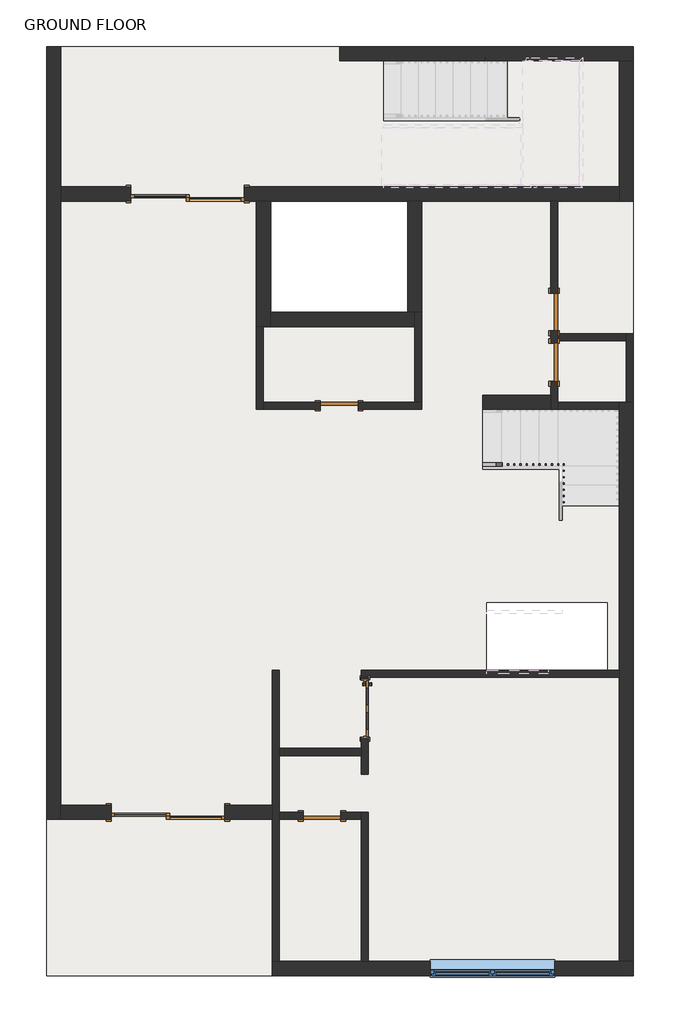
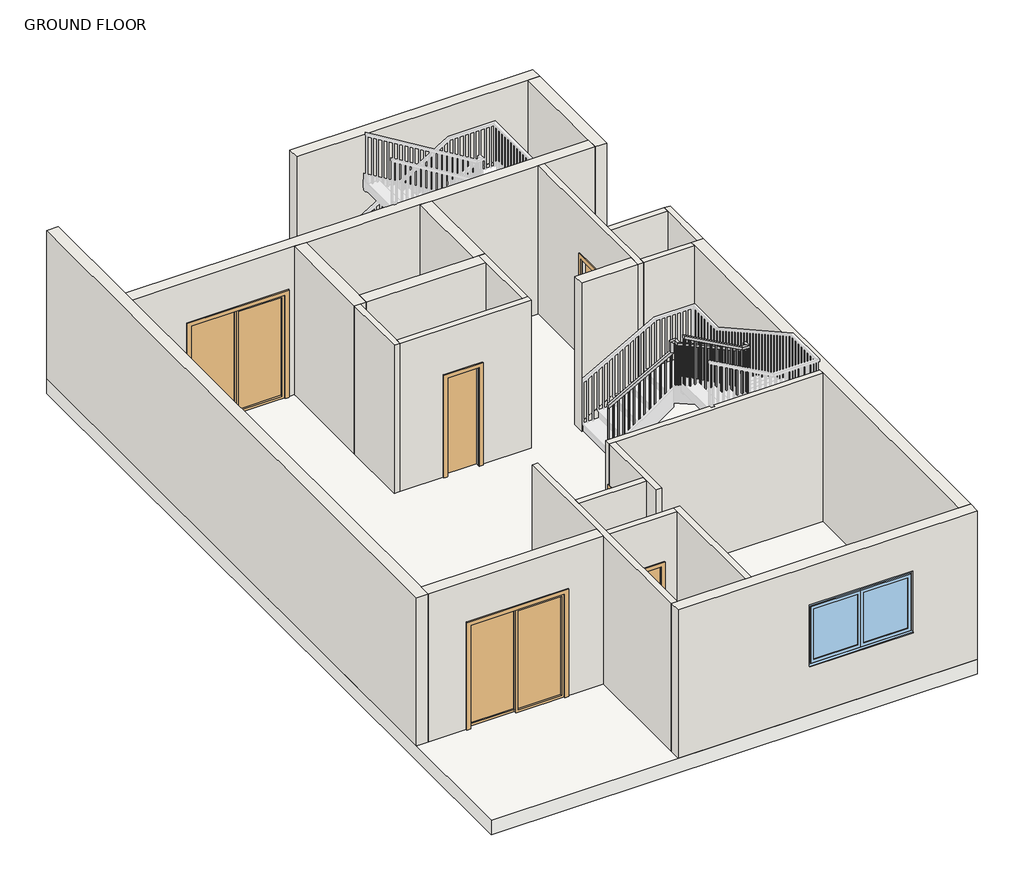
# One storey, part 1 of 3: 24 walls, 7 doors, 1 railing, 1 slab, 1 window.
"""IFC4 building model written with IfcOpenShell, lengths in millimetres."""

from ifc_helpers import new_model, si_unit, frame, origin, origin_with_axes, place, context, project, spatial, polyline, outline, extrude, faceted_brep, transform, mapped, element, save
from components import door_d4d75d1e, door_c2926031, single_flush_bathroom_door_2_x_7_d2bb450e, single_flush_bathroom_door_2_x_7_e2285e44, w2_w2_7b90d420

model = new_model("IFC4")

# Units and contexts
model_context = context("Model", 3, world=origin())
ifc_project = project(units=[si_unit("LENGTHUNIT", "METRE", prefix="MILLI")], contexts=[model_context])

# Site, building, storey
site = spatial("IfcSite", under=ifc_project)
building = spatial("IfcBuilding", under=site)
storey = spatial("IfcBuildingStorey", under=building, Name="GROUND FLOOR", Elevation=304.8)

# Doors
placement = place(None, origin())
door_shape = door_d4d75d1e(model_context)
element("IfcDoor", 1, ObjectType="Door-Double-Sliding : 72\" x 84\"", at=placement, inside=storey, context=model_context, shape_type="MappedRepresentation", body=[
    mapped(door_shape, transform((-16417.9229553, -4307.6035687, 304.8), x_axis=(-1.0, 0.0, 0.0), y_axis=(0.0, -1.0, 0.0), z_axis=(0.0, 0.0, 1.0))),
])
element("IfcDoor", 2, ObjectType="Door-Double-Sliding : 72\" x 84\"", at=placement, inside=storey, context=model_context, shape_type="MappedRepresentation", body=[
    mapped(door_shape, transform((-16100.4229553, 5649.1964313, 304.8), x_axis=(-1.0, 0.0, 0.0), y_axis=(0.0, -1.0, 0.0), z_axis=(0.0, 0.0, 1.0))),
])
door_2_shape = door_c2926031(model_context)
element("IfcDoor", 3, ObjectType="Door-Interior-Single-4_Panel-Wood : 36\" x 84\"", at=placement, inside=storey, context=model_context, shape_type="MappedRepresentation", body=[
    mapped(door_2_shape, transform((-13246.0979553, -2764.5535687, 304.8), x_axis=(0.0, -1.0, 0.0), y_axis=(1.0, 0.0, 0.0), z_axis=(0.0, 0.0, 1.0))),
])
single_flush_bathroom_door_2_x_7_shape = single_flush_bathroom_door_2_x_7_d2bb450e(model_context)
element("IfcDoor", 4, ObjectType="Single-Flush : BATHROOM DOOR 2' X 7'", at=placement, inside=storey, context=model_context, shape_type="MappedRepresentation", body=[
    mapped(single_flush_bathroom_door_2_x_7_shape, transform((-10201.2729553, 3623.5464313, 304.8), x_axis=(0.0, -1.0, 0.0), y_axis=(1.0, 0.0, 0.0), z_axis=(0.0, 0.0, 1.0))),
])
element("IfcDoor", 5, ObjectType="Single-Flush : BATHROOM DOOR 2' X 7'", at=placement, inside=storey, context=model_context, shape_type="MappedRepresentation", body=[
    mapped(single_flush_bathroom_door_2_x_7_shape, transform((-13938.2479553, -4491.7535687, 304.8), x_axis=(-1.0, 0.0, 0.0), y_axis=(0.0, -1.0, 0.0), z_axis=(0.0, 0.0, 1.0))),
])
element("IfcDoor", 6, ObjectType="Single-Flush : BATHROOM DOOR 2' X 7'", at=placement, inside=storey, context=model_context, shape_type="MappedRepresentation", body=[
    mapped(single_flush_bathroom_door_2_x_7_shape, transform((-13662.0229553, 2112.2464313, 304.8), x_axis=(1.0, 0.0, 0.0), y_axis=(0.0, 1.0, 0.0), z_axis=(0.0, 0.0, 1.0))),
])
single_flush_bathroom_door_2_x_7_2_shape = single_flush_bathroom_door_2_x_7_e2285e44(model_context)
element("IfcDoor", 7, ObjectType="Single-Flush : BATHROOM DOOR 2' X 7'", at=placement, inside=storey, context=model_context, shape_type="MappedRepresentation", body=[
    mapped(single_flush_bathroom_door_2_x_7_2_shape, transform((-10201.2729553, 2810.7464313, 304.8), x_axis=(0.0, 1.0, 0.0), y_axis=(-1.0, 0.0, 0.0), z_axis=(0.0, 0.0, 1.0))),
])

# Railing
element("IfcRailing", 8, ObjectType="Handrail - Rectangular", at=placement, inside=storey, context=model_context, shape_type="SolidModel", body=[
    faceted_brep([(-11350.6229553, 1191.4964313, 1388.5333333), (-11350.6229553, 1191.4964313, 1330.420221), (-11350.6229553, 1140.6964313, 1330.420221), (-11350.6229553, 1140.6964313, 1388.5333333), (-10144.1229553, 1191.4964313, 2058.8111111), (-10093.3229553, 1191.4964313, 2028.920221), (-10093.3229553, 1140.6964313, 2028.920221), (-10144.1229553, 1140.6964313, 2058.8111111), (-10144.1229553, 1191.4964313, 2277.5333333), (-10093.3229553, 1191.4964313, 2226.7333333), (-10093.3229553, 1140.6964313, 2226.7333333), (-10144.1229553, 1140.6964313, 2277.5333333), (-10017.1229553, 1191.4964313, 2277.5333333), (-10017.1229553, 1191.4964313, 2226.7333333), (-10067.9229553, 1140.6964313, 2226.7333333), (-10067.9229553, 1140.6964313, 2277.5333333), (-10017.1229553, 1064.4964313, 2277.5333333), (-10017.1229553, 1051.3328291, 2226.7333333), (-10067.9229553, 1051.3328291, 2226.7333333), (-10067.9229553, 1064.4964313, 2277.5333333), (-10017.1229553, -1158.0035687, 3512.2555556), (-10017.1229553, -1208.8035687, 3482.3646654), (-10067.9229553, -1208.8035687, 3482.3646654), (-10067.9229553, -1158.0035687, 3512.2555556), (-10017.1229553, -1158.0035687, 3632.2), (-10017.1229553, -1208.8035687, 3581.4), (-10067.9229553, -1208.8035687, 3581.4), (-10067.9229553, -1158.0035687, 3632.2), (-10017.1229553, -1285.0035687, 3632.2), (-10017.1229553, -1285.0035687, 3581.4), (-10067.9229553, -1234.2035687, 3581.4), (-10067.9229553, -1234.2035687, 3632.2), (-10144.1229553, -1285.0035687, 3632.2), (-10157.2865575, -1285.0035687, 3581.4), (-10157.2865575, -1234.2035687, 3581.4), (-10144.1229553, -1234.2035687, 3632.2), (-11287.1229553, -1285.0035687, 4267.2), (-11287.1229553, -1234.2035687, 4267.2), (-11287.1229553, -1234.2035687, 4209.0868876), (-11287.1229553, -1285.0035687, 4209.0868876)], [[[0, 1, 2, 3]], [[1, 0, 4, 5]], [[2, 1, 5, 6]], [[3, 2, 6, 7]], [[0, 3, 7, 4]], [[5, 4, 8, 9]], [[6, 5, 9, 10]], [[7, 6, 10, 11]], [[4, 7, 11, 8]], [[9, 8, 12, 13]], [[10, 9, 13, 14]], [[11, 10, 14, 15]], [[8, 11, 15, 12]], [[13, 12, 16, 17]], [[14, 13, 17, 18]], [[15, 14, 18, 19]], [[12, 15, 19, 16]], [[17, 16, 20, 21]], [[18, 17, 21, 22]], [[19, 18, 22, 23]], [[16, 19, 23, 20]], [[21, 20, 24, 25]], [[22, 21, 25, 26]], [[23, 22, 26, 27]], [[20, 23, 27, 24]], [[25, 24, 28, 29]], [[26, 25, 29, 30]], [[27, 26, 30, 31]], [[24, 27, 31, 28]], [[29, 28, 32, 33]], [[30, 29, 33, 34]], [[31, 30, 34, 35]], [[28, 31, 35, 32]], [[36, 37, 38, 39]], [[33, 32, 36, 39]], [[34, 33, 39, 38]], [[35, 34, 38, 37]], [[32, 35, 37, 36]]]),
    extrude(outline(polyline([(4189.6841099, -11252.1979553), (4200.2674432, -11271.2479553), (3183.4666667, -11271.2479553), (3183.4666667, -11252.1979553), (4189.6841099, -11252.1979553)])), frame((0.0, -1269.1285687, 0.0), z_axis=(0.0, 1.0, 0.0), x_axis=(0.0, 0.0, 1.0)), (0.0, 0.0, 1.0), 19.05),
    extrude(outline(polyline([(4133.2396654, -11150.5979553), (4143.8229988, -11169.6479553), (3183.4666667, -11169.6479553), (3183.4666667, -11150.5979553), (4133.2396654, -11150.5979553)])), frame((0.0, -1269.1285687, 0.0), z_axis=(0.0, 1.0, 0.0), x_axis=(0.0, 0.0, 1.0)), (0.0, 0.0, 1.0), 19.05),
    extrude(outline(polyline([(4076.795221, -11048.9979553), (4087.3785543, -11068.0479553), (3183.4666667, -11068.0479553), (3183.4666667, -11048.9979553), (4076.795221, -11048.9979553)])), frame((0.0, -1269.1285687, 0.0), z_axis=(0.0, 1.0, 0.0), x_axis=(0.0, 0.0, 1.0)), (0.0, 0.0, 1.0), 19.05),
    extrude(outline(polyline([(4020.3507765, -10947.3979553), (4030.9341099, -10966.4479553), (3014.1333333, -10966.4479553), (3014.1333333, -10947.3979553), (4020.3507765, -10947.3979553)])), frame((0.0, -1269.1285687, 0.0), z_axis=(0.0, 1.0, 0.0), x_axis=(0.0, 0.0, 1.0)), (0.0, 0.0, 1.0), 19.05),
    extrude(outline(polyline([(3963.9063321, -10845.7979553), (3974.4896654, -10864.8479553), (3014.1333333, -10864.8479553), (3014.1333333, -10845.7979553), (3963.9063321, -10845.7979553)])), frame((0.0, -1269.1285687, 0.0), z_axis=(0.0, 1.0, 0.0), x_axis=(0.0, 0.0, 1.0)), (0.0, 0.0, 1.0), 19.05),
    extrude(outline(polyline([(3907.4618876, -10744.1979553), (3918.045221, -10763.2479553), (3014.1333333, -10763.2479553), (3014.1333333, -10744.1979553), (3907.4618876, -10744.1979553)])), frame((0.0, -1269.1285687, 0.0), z_axis=(0.0, 1.0, 0.0), x_axis=(0.0, 0.0, 1.0)), (0.0, 0.0, 1.0), 19.05),
    extrude(outline(polyline([(3851.0174432, -10642.5979553), (3861.6007765, -10661.6479553), (2844.8, -10661.6479553), (2844.8, -10642.5979553), (3851.0174432, -10642.5979553)])), frame((0.0, -1269.1285687, 0.0), z_axis=(0.0, 1.0, 0.0), x_axis=(0.0, 0.0, 1.0)), (0.0, 0.0, 1.0), 19.05),
    extrude(outline(polyline([(3794.5729988, -10540.9979553), (3805.1563321, -10560.0479553), (2844.8, -10560.0479553), (2844.8, -10540.9979553), (3794.5729988, -10540.9979553)])), frame((0.0, -1269.1285687, 0.0), z_axis=(0.0, 1.0, 0.0), x_axis=(0.0, 0.0, 1.0)), (0.0, 0.0, 1.0), 19.05),
    extrude(outline(polyline([(3738.1285543, -10439.3979553), (3748.7118876, -10458.4479553), (2844.8, -10458.4479553), (2844.8, -10439.3979553), (3738.1285543, -10439.3979553)])), frame((0.0, -1269.1285687, 0.0), z_axis=(0.0, 1.0, 0.0), x_axis=(0.0, 0.0, 1.0)), (0.0, 0.0, 1.0), 19.05),
    extrude(outline(polyline([(3681.6841099, -10337.7979553), (3692.2674432, -10356.8479553), (2675.4666667, -10356.8479553), (2675.4666667, -10337.7979553), (3681.6841099, -10337.7979553)])), frame((0.0, -1269.1285687, 0.0), z_axis=(0.0, 1.0, 0.0), x_axis=(0.0, 0.0, 1.0)), (0.0, 0.0, 1.0), 19.05),
    extrude(outline(polyline([(3625.2396654, -10236.1979553), (3635.8229988, -10255.2479553), (2675.4666667, -10255.2479553), (2675.4666667, -10236.1979553), (3625.2396654, -10236.1979553)])), frame((0.0, -1269.1285687, 0.0), z_axis=(0.0, 1.0, 0.0), x_axis=(0.0, 0.0, 1.0)), (0.0, 0.0, 1.0), 19.05),
    extrude(outline(polyline([(3568.795221, -10134.5979553), (3579.3785543, -10153.6479553), (2675.4666667, -10153.6479553), (2675.4666667, -10134.5979553), (3568.795221, -10134.5979553)])), frame((0.0, -1269.1285687, 0.0), z_axis=(0.0, 1.0, 0.0), x_axis=(0.0, 0.0, 1.0)), (0.0, 0.0, 1.0), 19.05),
    extrude(outline(polyline([(-10052.0479553, -1161.1785687), (-10032.9979553, -1161.1785687), (-10032.9979553, -1180.2285687), (-10052.0479553, -1180.2285687), (-10052.0479553, -1161.1785687)])), frame((0.0, 0.0, 2506.1333333), z_axis=(0.0, 0.0, 1.0), x_axis=(1.0, 0.0, 0.0)), (0.0, 0.0, 1.0), 1075.2666667),
    extrude(outline(polyline([(-1078.6285687, 3410.045221), (-1059.5785687, 3399.4618876), (-1059.5785687, 2506.1333333), (-1078.6285687, 2506.1333333), (-1078.6285687, 3410.045221)])), frame((-10052.0479553, 0.0, 0.0), z_axis=(1.0, 0.0, 0.0), x_axis=(0.0, 1.0, 0.0)), (0.0, 0.0, 1.0), 19.05),
    extrude(outline(polyline([(-977.0285687, 3353.6007765), (-957.9785687, 3343.0174432), (-957.9785687, 2336.8), (-977.0285687, 2336.8), (-977.0285687, 3353.6007765)])), frame((-10052.0479553, 0.0, 0.0), z_axis=(1.0, 0.0, 0.0), x_axis=(0.0, 1.0, 0.0)), (0.0, 0.0, 1.0), 19.05),
    extrude(outline(polyline([(-875.4285687, 3297.1563321), (-856.3785687, 3286.5729988), (-856.3785687, 2336.8), (-875.4285687, 2336.8), (-875.4285687, 3297.1563321)])), frame((-10052.0479553, 0.0, 0.0), z_axis=(1.0, 0.0, 0.0), x_axis=(0.0, 1.0, 0.0)), (0.0, 0.0, 1.0), 19.05),
    extrude(outline(polyline([(-773.8285687, 3240.7118876), (-754.7785687, 3230.1285543), (-754.7785687, 2336.8), (-773.8285687, 2336.8), (-773.8285687, 3240.7118876)])), frame((-10052.0479553, 0.0, 0.0), z_axis=(1.0, 0.0, 0.0), x_axis=(0.0, 1.0, 0.0)), (0.0, 0.0, 1.0), 19.05),
    extrude(outline(polyline([(-672.2285687, 3184.2674432), (-653.1785687, 3173.6841099), (-653.1785687, 2167.4666667), (-672.2285687, 2167.4666667), (-672.2285687, 3184.2674432)])), frame((-10052.0479553, 0.0, 0.0), z_axis=(1.0, 0.0, 0.0), x_axis=(0.0, 1.0, 0.0)), (0.0, 0.0, 1.0), 19.05),
    extrude(outline(polyline([(-570.6285687, 3127.8229988), (-551.5785687, 3117.2396654), (-551.5785687, 2167.4666667), (-570.6285687, 2167.4666667), (-570.6285687, 3127.8229988)])), frame((-10052.0479553, 0.0, 0.0), z_axis=(1.0, 0.0, 0.0), x_axis=(0.0, 1.0, 0.0)), (0.0, 0.0, 1.0), 19.05),
    extrude(outline(polyline([(-469.0285687, 3071.3785543), (-449.9785687, 3060.795221), (-449.9785687, 2167.4666667), (-469.0285687, 2167.4666667), (-469.0285687, 3071.3785543)])), frame((-10052.0479553, 0.0, 0.0), z_axis=(1.0, 0.0, 0.0), x_axis=(0.0, 1.0, 0.0)), (0.0, 0.0, 1.0), 19.05),
    extrude(outline(polyline([(-367.4285687, 3014.9341099), (-348.3785687, 3004.3507765), (-348.3785687, 1998.1333333), (-367.4285687, 1998.1333333), (-367.4285687, 3014.9341099)])), frame((-10052.0479553, 0.0, 0.0), z_axis=(1.0, 0.0, 0.0), x_axis=(0.0, 1.0, 0.0)), (0.0, 0.0, 1.0), 19.05),
    extrude(outline(polyline([(-265.8285687, 2958.4896654), (-246.7785687, 2947.9063321), (-246.7785687, 1998.1333333), (-265.8285687, 1998.1333333), (-265.8285687, 2958.4896654)])), frame((-10052.0479553, 0.0, 0.0), z_axis=(1.0, 0.0, 0.0), x_axis=(0.0, 1.0, 0.0)), (0.0, 0.0, 1.0), 19.05),
    extrude(outline(polyline([(-164.2285687, 2902.045221), (-145.1785687, 2891.4618876), (-145.1785687, 1998.1333333), (-164.2285687, 1998.1333333), (-164.2285687, 2902.045221)])), frame((-10052.0479553, 0.0, 0.0), z_axis=(1.0, 0.0, 0.0), x_axis=(0.0, 1.0, 0.0)), (0.0, 0.0, 1.0), 19.05),
    extrude(outline(polyline([(-62.6285687, 2845.6007765), (-43.5785687, 2835.0174432), (-43.5785687, 1828.8), (-62.6285687, 1828.8), (-62.6285687, 2845.6007765)])), frame((-10052.0479553, 0.0, 0.0), z_axis=(1.0, 0.0, 0.0), x_axis=(0.0, 1.0, 0.0)), (0.0, 0.0, 1.0), 19.05),
    extrude(outline(polyline([(38.9714313, 2789.1563321), (58.0214313, 2778.5729988), (58.0214313, 1828.8), (38.9714313, 1828.8), (38.9714313, 2789.1563321)])), frame((-10052.0479553, 0.0, 0.0), z_axis=(1.0, 0.0, 0.0), x_axis=(0.0, 1.0, 0.0)), (0.0, 0.0, 1.0), 19.05),
    extrude(outline(polyline([(140.5714313, 2732.7118876), (159.6214313, 2722.1285543), (159.6214313, 1828.8), (140.5714313, 1828.8), (140.5714313, 2732.7118876)])), frame((-10052.0479553, 0.0, 0.0), z_axis=(1.0, 0.0, 0.0), x_axis=(0.0, 1.0, 0.0)), (0.0, 0.0, 1.0), 19.05),
    extrude(outline(polyline([(242.1714313, 2676.2674432), (261.2214313, 2665.6841099), (261.2214313, 1659.4666667), (242.1714313, 1659.4666667), (242.1714313, 2676.2674432)])), frame((-10052.0479553, 0.0, 0.0), z_axis=(1.0, 0.0, 0.0), x_axis=(0.0, 1.0, 0.0)), (0.0, 0.0, 1.0), 19.05),
    extrude(outline(polyline([(343.7714313, 2619.8229988), (362.8214313, 2609.2396654), (362.8214313, 1659.4666667), (343.7714313, 1659.4666667), (343.7714313, 2619.8229988)])), frame((-10052.0479553, 0.0, 0.0), z_axis=(1.0, 0.0, 0.0), x_axis=(0.0, 1.0, 0.0)), (0.0, 0.0, 1.0), 19.05),
    extrude(outline(polyline([(445.3714313, 2563.3785543), (464.4214313, 2552.795221), (464.4214313, 1659.4666667), (445.3714313, 1659.4666667), (445.3714313, 2563.3785543)])), frame((-10052.0479553, 0.0, 0.0), z_axis=(1.0, 0.0, 0.0), x_axis=(0.0, 1.0, 0.0)), (0.0, 0.0, 1.0), 19.05),
    extrude(outline(polyline([(546.9714313, 2506.9341099), (566.0214313, 2496.3507765), (566.0214313, 1490.1333333), (546.9714313, 1490.1333333), (546.9714313, 2506.9341099)])), frame((-10052.0479553, 0.0, 0.0), z_axis=(1.0, 0.0, 0.0), x_axis=(0.0, 1.0, 0.0)), (0.0, 0.0, 1.0), 19.05),
    extrude(outline(polyline([(648.5714313, 2450.4896654), (667.6214313, 2439.9063321), (667.6214313, 1490.1333333), (648.5714313, 1490.1333333), (648.5714313, 2450.4896654)])), frame((-10052.0479553, 0.0, 0.0), z_axis=(1.0, 0.0, 0.0), x_axis=(0.0, 1.0, 0.0)), (0.0, 0.0, 1.0), 19.05),
    extrude(outline(polyline([(750.1714313, 2394.045221), (769.2214313, 2383.4618876), (769.2214313, 1490.1333333), (750.1714313, 1490.1333333), (750.1714313, 2394.045221)])), frame((-10052.0479553, 0.0, 0.0), z_axis=(1.0, 0.0, 0.0), x_axis=(0.0, 1.0, 0.0)), (0.0, 0.0, 1.0), 19.05),
    extrude(outline(polyline([(851.7714313, 2337.6007765), (870.8214313, 2327.0174432), (870.8214313, 1320.8), (851.7714313, 1320.8), (851.7714313, 2337.6007765)])), frame((-10052.0479553, 0.0, 0.0), z_axis=(1.0, 0.0, 0.0), x_axis=(0.0, 1.0, 0.0)), (0.0, 0.0, 1.0), 19.05),
    extrude(outline(polyline([(953.3714313, 2281.1563321), (972.4214313, 2270.5729988), (972.4214313, 1320.8), (953.3714313, 1320.8), (953.3714313, 2281.1563321)])), frame((-10052.0479553, 0.0, 0.0), z_axis=(1.0, 0.0, 0.0), x_axis=(0.0, 1.0, 0.0)), (0.0, 0.0, 1.0), 19.05),
    extrude(outline(polyline([(1054.9714313, 2224.7118876), (1074.0214313, 2214.1285543), (1074.0214313, 1320.8), (1054.9714313, 1320.8), (1054.9714313, 2224.7118876)])), frame((-10052.0479553, 0.0, 0.0), z_axis=(1.0, 0.0, 0.0), x_axis=(0.0, 1.0, 0.0)), (0.0, 0.0, 1.0), 19.05),
    extrude(outline(polyline([(-10140.9479553, 1156.5714313), (-10140.9479553, 1175.6214313), (-10121.8979553, 1175.6214313), (-10121.8979553, 1156.5714313), (-10140.9479553, 1156.5714313)])), frame((0.0, 0.0, 1151.4666667), z_axis=(0.0, 0.0, 1.0), x_axis=(1.0, 0.0, 0.0)), (0.0, 0.0, 1.0), 1075.2666667),
    extrude(outline(polyline([(1956.6007765, -10223.4979553), (1946.0174432, -10242.5479553), (982.1333333, -10242.5479553), (982.1333333, -10223.4979553), (1956.6007765, -10223.4979553)])), frame((0.0, 1156.5714313, 0.0), z_axis=(0.0, 1.0, 0.0), x_axis=(0.0, 0.0, 1.0)), (0.0, 0.0, 1.0), 19.05),
    extrude(outline(polyline([(1900.1563321, -10325.0979553), (1889.5729988, -10344.1479553), (982.1333333, -10344.1479553), (982.1333333, -10325.0979553), (1900.1563321, -10325.0979553)])), frame((0.0, 1156.5714313, 0.0), z_axis=(0.0, 1.0, 0.0), x_axis=(0.0, 0.0, 1.0)), (0.0, 0.0, 1.0), 19.05),
    extrude(outline(polyline([(1843.7118876, -10426.6979553), (1833.1285543, -10445.7479553), (982.1333333, -10445.7479553), (982.1333333, -10426.6979553), (1843.7118876, -10426.6979553)])), frame((0.0, 1156.5714313, 0.0), z_axis=(0.0, 1.0, 0.0), x_axis=(0.0, 0.0, 1.0)), (0.0, 0.0, 1.0), 19.05),
    extrude(outline(polyline([(1787.2674432, -10528.2979553), (1776.6841099, -10547.3479553), (812.8, -10547.3479553), (812.8, -10528.2979553), (1787.2674432, -10528.2979553)])), frame((0.0, 1156.5714313, 0.0), z_axis=(0.0, 1.0, 0.0), x_axis=(0.0, 0.0, 1.0)), (0.0, 0.0, 1.0), 19.05),
    extrude(outline(polyline([(1730.8229988, -10629.8979553), (1720.2396654, -10648.9479553), (812.8, -10648.9479553), (812.8, -10629.8979553), (1730.8229988, -10629.8979553)])), frame((0.0, 1156.5714313, 0.0), z_axis=(0.0, 1.0, 0.0), x_axis=(0.0, 0.0, 1.0)), (0.0, 0.0, 1.0), 19.05),
    extrude(outline(polyline([(1674.3785543, -10731.4979553), (1663.795221, -10750.5479553), (812.8, -10750.5479553), (812.8, -10731.4979553), (1674.3785543, -10731.4979553)])), frame((0.0, 1156.5714313, 0.0), z_axis=(0.0, 1.0, 0.0), x_axis=(0.0, 0.0, 1.0)), (0.0, 0.0, 1.0), 19.05),
    extrude(outline(polyline([(1617.9341099, -10833.0979553), (1607.3507765, -10852.1479553), (643.4666667, -10852.1479553), (643.4666667, -10833.0979553), (1617.9341099, -10833.0979553)])), frame((0.0, 1156.5714313, 0.0), z_axis=(0.0, 1.0, 0.0), x_axis=(0.0, 0.0, 1.0)), (0.0, 0.0, 1.0), 19.05),
    extrude(outline(polyline([(1561.4896654, -10934.6979553), (1550.9063321, -10953.7479553), (643.4666667, -10953.7479553), (643.4666667, -10934.6979553), (1561.4896654, -10934.6979553)])), frame((0.0, 1156.5714313, 0.0), z_axis=(0.0, 1.0, 0.0), x_axis=(0.0, 0.0, 1.0)), (0.0, 0.0, 1.0), 19.05),
    extrude(outline(polyline([(1505.045221, -11036.2979553), (1494.4618876, -11055.3479553), (643.4666667, -11055.3479553), (643.4666667, -11036.2979553), (1505.045221, -11036.2979553)])), frame((0.0, 1156.5714313, 0.0), z_axis=(0.0, 1.0, 0.0), x_axis=(0.0, 0.0, 1.0)), (0.0, 0.0, 1.0), 19.05),
    extrude(outline(polyline([(1448.6007765, -11137.8979553), (1438.0174432, -11156.9479553), (474.1333333, -11156.9479553), (474.1333333, -11137.8979553), (1448.6007765, -11137.8979553)])), frame((0.0, 1156.5714313, 0.0), z_axis=(0.0, 1.0, 0.0), x_axis=(0.0, 0.0, 1.0)), (0.0, 0.0, 1.0), 19.05),
    extrude(outline(polyline([(1392.1563321, -11239.4979553), (1381.5729988, -11258.5479553), (474.1333333, -11258.5479553), (474.1333333, -11239.4979553), (1392.1563321, -11239.4979553)])), frame((0.0, 1156.5714313, 0.0), z_axis=(0.0, 1.0, 0.0), x_axis=(0.0, 0.0, 1.0)), (0.0, 0.0, 1.0), 19.05),
    extrude(outline(polyline([(-10052.0479553, -1250.0785687), (-10032.9979553, -1250.0785687), (-10032.9979553, -1269.1285687), (-10052.0479553, -1269.1285687), (-10052.0479553, -1250.0785687)])), frame((0.0, 0.0, 2506.1333333), z_axis=(0.0, 0.0, 1.0), x_axis=(1.0, 0.0, 0.0)), (0.0, 0.0, 1.0), 1075.2666667),
    extrude(outline(polyline([(-10052.0479553, 1156.5714313), (-10052.0479553, 1175.6214313), (-10032.9979553, 1175.6214313), (-10032.9979553, 1156.5714313), (-10052.0479553, 1156.5714313)])), frame((0.0, 0.0, 1151.4666667), z_axis=(0.0, 0.0, 1.0), x_axis=(1.0, 0.0, 0.0)), (0.0, 0.0, 1.0), 1075.2666667),
    extrude(outline(polyline([(4198.5035543, -11268.0729553), (4209.0868876, -11287.1229553), (3183.4666667, -11287.1229553), (3183.4666667, -11268.0729553), (4198.5035543, -11268.0729553)])), frame((0.0, -1269.1285687, 0.0), z_axis=(0.0, 1.0, 0.0), x_axis=(0.0, 0.0, 1.0)), (0.0, 0.0, 1.0), 19.05),
    extrude(outline(polyline([(1341.0035543, -11331.5729553), (1330.420221, -11350.6229553), (474.1333333, -11350.6229553), (474.1333333, -11331.5729553), (1341.0035543, -11331.5729553)])), frame((0.0, 1156.5714313, 0.0), z_axis=(0.0, 1.0, 0.0), x_axis=(0.0, 0.0, 1.0)), (0.0, 0.0, 1.0), 19.05),
])

# Slab
element("IfcSlab", 9, at=placement, inside=storey, context=model_context, shape_type="SweptSolid", body=[
    extrude(outline(polyline([(-8924.9229553, 7897.0964313), (-8924.9229553, -7063.5035687), (-18373.7229553, -7063.5035687), (-18373.7229553, 7897.0964313), (-8924.9229553, 7897.0964313)]), holes=[polyline([(-12557.1229553, 5407.8964313), (-14766.9229553, 5407.8964313), (-14766.9229553, 3617.1964313), (-12557.1229553, 3617.1964313), (-12557.1229553, 5407.8964313)]), polyline([(-11287.1229553, -2148.6035687), (-9344.0229553, -2148.6035687), (-9344.0229553, -1056.4035687), (-11287.1229553, -1056.4035687), (-11287.1229553, -2148.6035687)])]), origin_with_axes(), (0.0, 0.0, 1.0), 304.8),
])

# Walls
element("IfcWall", 10, ObjectType="EXTERIOR WALL 9\"", at=placement, inside=storey, context=model_context, shape_type="Brep", body=[
    faceted_brep([(-13649.3229553, 7668.4964313, 304.8), (-9153.5229553, 7668.4964313, 304.8), (-8924.9229553, 7668.4964313, 304.8), (-8924.9229553, 7668.4964313, 3352.8), (-9153.5229553, 7668.4964313, 3352.8), (-13649.3229553, 7668.4964313, 3352.8), (-13649.3229553, 7897.0964313, 304.8), (-13649.3229553, 7897.0964313, 3352.8), (-8924.9229553, 7897.0964313, 3352.8), (-8924.9229553, 7897.0964313, 304.8)], [[[0, 1, 2, 3, 4, 5]], [[6, 7, 8, 9]], [[2, 1, 0, 6, 9]], [[5, 4, 3, 8, 7]], [[0, 5, 7, 6]], [[3, 2, 9, 8]]]),
])
element("IfcWall", 11, ObjectType="EXTERIOR WALL 9\"", at=placement, inside=storey, context=model_context, shape_type="Brep", body=[
    faceted_brep([(-9153.5229553, 7668.4964313, 304.8), (-9153.5229553, 5636.4964313, 304.8), (-9153.5229553, 5407.8964313, 304.8), (-9153.5229553, 5407.8964313, 3352.8), (-9153.5229553, 5636.4964313, 3352.8), (-9153.5229553, 7668.4964313, 3352.8), (-8924.9229553, 7668.4964313, 304.8), (-8924.9229553, 7668.4964313, 3352.8), (-8924.9229553, 5407.8964313, 3352.8), (-8924.9229553, 5407.8964313, 304.8)], [[[0, 1, 2, 3, 4, 5]], [[6, 7, 8, 9]], [[2, 1, 0, 6, 9]], [[5, 4, 3, 8, 7]], [[0, 5, 7, 6]], [[3, 2, 9, 8]]]),
])
element("IfcWall", 12, ObjectType="EXTERIOR WALL 9\"", at=placement, inside=storey, context=model_context, shape_type="Brep", body=[
    faceted_brep([(-17014.8229553, 5636.4964313, 2438.4), (-17014.8229553, 5636.4964313, 304.8), (-18145.1229553, 5636.4964313, 304.8), (-18145.1229553, 5636.4964313, 3352.8), (-9153.5229553, 5636.4964313, 3352.8), (-9153.5229553, 5636.4964313, 304.8), (-15186.0229553, 5636.4964313, 304.8), (-15186.0229553, 5636.4964313, 2438.4), (-18145.1229553, 5407.8964313, 304.8), (-17014.8229553, 5407.8964313, 304.8), (-17014.8229553, 5407.8964313, 2438.4), (-15186.0229553, 5407.8964313, 2438.4), (-15186.0229553, 5407.8964313, 304.8), (-14995.5229553, 5407.8964313, 304.8), (-14766.9229553, 5407.8964313, 304.8), (-12557.1229553, 5407.8964313, 304.8), (-12328.5229553, 5407.8964313, 304.8), (-10258.4229553, 5407.8964313, 304.8), (-10144.1229553, 5407.8964313, 304.8), (-9153.5229553, 5407.8964313, 304.8), (-9153.5229553, 5407.8964313, 3352.8), (-10144.1229553, 5407.8964313, 3352.8), (-10258.4229553, 5407.8964313, 3352.8), (-12328.5229553, 5407.8964313, 3352.8), (-12557.1229553, 5407.8964313, 3352.8), (-14766.9229553, 5407.8964313, 3352.8), (-14995.5229553, 5407.8964313, 3352.8), (-18145.1229553, 5407.8964313, 3352.8)], [[[0, 1, 2, 3, 4, 5, 6, 7]], [[8, 9, 10, 11, 12, 13, 14, 15, 16, 17, 18, 19, 20, 21, 22, 23, 24, 25, 26, 27]], [[6, 5, 19, 18, 17, 16, 15, 14, 13, 12]], [[2, 1, 9, 8]], [[4, 3, 27, 26, 25, 24, 23, 22, 21, 20]], [[5, 4, 20, 19]], [[3, 2, 8, 27]], [[12, 11, 7, 6]], [[10, 9, 1, 0]], [[11, 10, 0, 7]]]),
])
element("IfcWall", 13, ObjectType="EXTERIOR WALL 9\"", at=placement, inside=storey, context=model_context, shape_type="Brep", body=[
    faceted_brep([(-18145.1229553, -4548.9035687, 304.8), (-18145.1229553, -4320.3035687, 304.8), (-18145.1229553, 5407.8964313, 304.8), (-18145.1229553, 5636.4964313, 304.8), (-18145.1229553, 7897.0964313, 304.8), (-18145.1229553, 7897.0964313, 3352.8), (-18145.1229553, 5636.4964313, 3352.8), (-18145.1229553, 5407.8964313, 3352.8), (-18145.1229553, -4320.3035687, 3352.8), (-18145.1229553, -4548.9035687, 3352.8), (-18373.7229553, -4548.9035687, 304.8), (-18373.7229553, -4548.9035687, 3352.8), (-18373.7229553, 7897.0964313, 3352.8), (-18373.7229553, 7897.0964313, 304.8)], [[[0, 1, 2, 3, 4, 5, 6, 7, 8, 9]], [[10, 11, 12, 13]], [[4, 3, 2, 1, 0, 10, 13]], [[5, 4, 13, 12]], [[9, 8, 7, 6, 5, 12, 11]], [[0, 9, 11, 10]]]),
])
element("IfcWall", 14, ObjectType="EXTERIOR WALL 9\"", at=placement, inside=storey, context=model_context, shape_type="SweptSolid", body=[
    extrude(outline(polyline([(304.8, -18145.1229553), (304.8, -17332.3229553), (2438.4, -17332.3229553), (2438.4, -15503.5229553), (304.8, -15503.5229553), (304.8, -14741.5229553), (3352.8, -14741.5229553), (3352.8, -18145.1229553), (304.8, -18145.1229553)])), frame((0.0, -4548.9035687, 0.0), z_axis=(0.0, 1.0, 0.0), x_axis=(0.0, 0.0, 1.0)), (0.0, 0.0, 1.0), 228.6),
])
element("IfcWall", 15, ObjectType="EXTERIOR WALL 9\"", at=placement, inside=storey, context=model_context, shape_type="Brep", body=[
    faceted_brep([(-14741.5229553, -7063.5035687, 304.8), (-8924.9229553, -7063.5035687, 304.8), (-8924.9229553, -7063.5035687, 3352.8), (-14741.5229553, -7063.5035687, 3352.8), (-12196.8729553, -7063.5035687, 1304.8), (-12196.8729553, -7063.5035687, 2564.8), (-10186.8729553, -7063.5035687, 2564.8), (-10186.8729553, -7063.5035687, 1304.8), (-14741.5229553, -6834.9035687, 304.8), (-14741.5229553, -6834.9035687, 3352.8), (-14627.2229553, -6834.9035687, 3352.8), (-13306.4229553, -6834.9035687, 3352.8), (-13192.1229553, -6834.9035687, 3352.8), (-9153.5229553, -6834.9035687, 3352.8), (-8924.9229553, -6834.9035687, 3352.8), (-8924.9229553, -6834.9035687, 304.8), (-9153.5229553, -6834.9035687, 304.8), (-13192.1229553, -6834.9035687, 304.8), (-13306.4229553, -6834.9035687, 304.8), (-14627.2229553, -6834.9035687, 304.8), (-12196.8729553, -6834.9035687, 1304.8), (-10186.8729553, -6834.9035687, 1304.8), (-10186.8729553, -6834.9035687, 2564.8), (-12196.8729553, -6834.9035687, 2564.8)], [[[0, 1, 2, 3], [4, 5, 6, 7]], [[8, 9, 10, 11, 12, 13, 14, 15, 16, 17, 18, 19], [20, 21, 22, 23]], [[1, 0, 8, 19, 18, 17, 16, 15]], [[3, 2, 14, 13, 12, 11, 10, 9]], [[2, 1, 15, 14]], [[0, 3, 9, 8]], [[5, 4, 20, 23]], [[6, 5, 23, 22]], [[7, 6, 22, 21]], [[4, 7, 21, 20]]]),
])
element("IfcWall", 16, ObjectType="EXTERIOR WALL 9\"", at=placement, inside=storey, context=model_context, shape_type="Brep", body=[
    faceted_brep([(-8924.9229553, -6834.9035687, 304.8), (-8924.9229553, 2169.3964313, 304.8), (-8924.9229553, 2169.3964313, 3352.8), (-8924.9229553, -6834.9035687, 3352.8), (-9153.5229553, -6834.9035687, 304.8), (-9153.5229553, -6834.9035687, 3352.8), (-9153.5229553, -2262.9035687, 3352.8), (-9153.5229553, -2148.6035687, 3352.8), (-9153.5229553, 2055.0964313, 3352.8), (-9153.5229553, 2169.3964313, 3352.8), (-9153.5229553, 2169.3964313, 304.8), (-9153.5229553, 2055.0964313, 304.8), (-9153.5229553, -2148.6035687, 304.8), (-9153.5229553, -2262.9035687, 304.8), (-9039.2229553, 2169.3964313, 304.8), (-9039.2229553, 2169.3964313, 3352.8)], [[[0, 1, 2, 3]], [[4, 5, 6, 7, 8, 9, 10, 11, 12, 13]], [[1, 0, 4, 13, 12, 11, 10, 14]], [[3, 2, 15, 9, 8, 7, 6, 5]], [[0, 3, 5, 4]], [[2, 1, 14, 10, 9, 15]]]),
])
element("IfcWall", 17, ObjectType="EXTERIOR WALL 9\"", at=placement, inside=storey, context=model_context, shape_type="SweptSolid", body=[
    extrude(outline(polyline([(-10258.4229553, 2055.0964313), (-11350.6229553, 2055.0964313), (-11350.6229553, 2283.6964313), (-10258.4229553, 2283.6964313), (-10258.4229553, 2055.0964313)])), frame((0.0, 0.0, 304.8), z_axis=(0.0, 0.0, 1.0), x_axis=(1.0, 0.0, 0.0)), (0.0, 0.0, 1.0), 3048.0),
])
element("IfcWall", 18, ObjectType="EXTERIOR WALL 9\"", at=placement, inside=storey, context=model_context, shape_type="Brep", body=[
    faceted_brep([(-14995.5229553, 5407.8964313, 304.8), (-14995.5229553, 3388.5964313, 304.8), (-14995.5229553, 3388.5964313, 3352.8), (-14995.5229553, 5407.8964313, 3352.8), (-14766.9229553, 5407.8964313, 304.8), (-14766.9229553, 5407.8964313, 3352.8), (-14766.9229553, 3617.1964313, 3352.8), (-14766.9229553, 3388.5964313, 3352.8), (-14766.9229553, 3388.5964313, 304.8), (-14766.9229553, 3617.1964313, 304.8), (-14881.2229553, 3388.5964313, 304.8), (-14881.2229553, 3388.5964313, 3352.8)], [[[0, 1, 2, 3]], [[4, 5, 6, 7, 8, 9]], [[1, 0, 4, 9, 8, 10]], [[3, 2, 11, 7, 6, 5]], [[0, 3, 5, 4]], [[2, 1, 10, 8, 7, 11]]]),
])
element("IfcWall", 19, ObjectType="EXTERIOR WALL 9\"", at=placement, inside=storey, context=model_context, shape_type="Brep", body=[
    faceted_brep([(-14766.9229553, 3388.5964313, 304.8), (-12442.8229553, 3388.5964313, 304.8), (-12442.8229553, 3388.5964313, 3352.8), (-14766.9229553, 3388.5964313, 3352.8), (-14766.9229553, 3617.1964313, 304.8), (-14766.9229553, 3617.1964313, 3352.8), (-12557.1229553, 3617.1964313, 3352.8), (-12442.8229553, 3617.1964313, 3352.8), (-12442.8229553, 3617.1964313, 304.8), (-12557.1229553, 3617.1964313, 304.8)], [[[0, 1, 2, 3]], [[4, 5, 6, 7, 8, 9]], [[1, 0, 4, 9, 8]], [[3, 2, 7, 6, 5]], [[0, 3, 5, 4]], [[2, 1, 8, 7]]]),
])
element("IfcWall", 20, ObjectType="EXTERIOR WALL 9\"", at=placement, inside=storey, context=model_context, shape_type="Brep", body=[
    faceted_brep([(-12557.1229553, 5407.8964313, 304.8), (-12557.1229553, 3617.1964313, 304.8), (-12557.1229553, 3617.1964313, 3352.8), (-12557.1229553, 5407.8964313, 3352.8), (-12328.5229553, 5407.8964313, 304.8), (-12328.5229553, 5407.8964313, 3352.8), (-12328.5229553, 3617.1964313, 3352.8), (-12328.5229553, 3617.1964313, 304.8), (-12442.8229553, 3617.1964313, 304.8), (-12442.8229553, 3617.1964313, 3352.8)], [[[0, 1, 2, 3]], [[4, 5, 6, 7]], [[1, 0, 4, 7, 8]], [[3, 2, 9, 6, 5]], [[2, 1, 8, 7, 6, 9]], [[0, 3, 5, 4]]]),
])
element("IfcWall", 21, ObjectType="INTERIOR WALL 4.5\"", at=placement, inside=storey, context=model_context, shape_type="Brep", body=[
    faceted_brep([(-14995.5229553, 3388.5964313, 304.8), (-14995.5229553, 2055.0964313, 304.8), (-14995.5229553, 2055.0964313, 3352.8), (-14995.5229553, 3388.5964313, 3352.8), (-14881.2229553, 3388.5964313, 304.8), (-14881.2229553, 3388.5964313, 3352.8), (-14881.2229553, 2169.3964313, 3352.8), (-14881.2229553, 2055.0964313, 3352.8), (-14881.2229553, 2055.0964313, 304.8), (-14881.2229553, 2169.3964313, 304.8)], [[[0, 1, 2, 3]], [[4, 5, 6, 7, 8, 9]], [[1, 0, 4, 9, 8]], [[3, 2, 7, 6, 5]], [[2, 1, 8, 7]], [[0, 3, 5, 4]]]),
])
element("IfcWall", 22, ObjectType="INTERIOR WALL 4.5\"", at=placement, inside=storey, context=model_context, shape_type="Brep", body=[
    faceted_brep([(-13357.2229553, 2055.0964313, 2336.8), (-13357.2229553, 2055.0964313, 304.8), (-12328.5229553, 2055.0964313, 304.8), (-12328.5229553, 2055.0964313, 3352.8), (-14881.2229553, 2055.0964313, 3352.8), (-14881.2229553, 2055.0964313, 304.8), (-13966.8229553, 2055.0964313, 304.8), (-13966.8229553, 2055.0964313, 2336.8), (-12328.5229553, 2169.3964313, 304.8), (-12442.8229553, 2169.3964313, 304.8), (-13357.2229553, 2169.3964313, 304.8), (-13357.2229553, 2169.3964313, 2336.8), (-13966.8229553, 2169.3964313, 2336.8), (-13966.8229553, 2169.3964313, 304.8), (-14881.2229553, 2169.3964313, 304.8), (-14881.2229553, 2169.3964313, 3352.8), (-12442.8229553, 2169.3964313, 3352.8), (-12328.5229553, 2169.3964313, 3352.8)], [[[0, 1, 2, 3, 4, 5, 6, 7]], [[8, 9, 10, 11, 12, 13, 14, 15, 16, 17]], [[6, 5, 14, 13]], [[2, 1, 10, 9, 8]], [[4, 3, 17, 16, 15]], [[5, 4, 15, 14]], [[3, 2, 8, 17]], [[11, 10, 1, 0]], [[12, 11, 0, 7]], [[13, 12, 7, 6]]]),
])
element("IfcWall", 23, ObjectType="INTERIOR WALL 4.5\"", at=placement, inside=storey, context=model_context, shape_type="Brep", body=[
    faceted_brep([(-12328.5229553, 2169.3964313, 304.8), (-12328.5229553, 3617.1964313, 304.8), (-12328.5229553, 3617.1964313, 3352.8), (-12328.5229553, 2169.3964313, 3352.8), (-12442.8229553, 2169.3964313, 304.8), (-12442.8229553, 2169.3964313, 3352.8), (-12442.8229553, 3388.5964313, 3352.8), (-12442.8229553, 3617.1964313, 3352.8), (-12442.8229553, 3617.1964313, 304.8), (-12442.8229553, 3388.5964313, 304.8)], [[[0, 1, 2, 3]], [[4, 5, 6, 7, 8, 9]], [[1, 0, 4, 9, 8]], [[3, 2, 7, 6, 5]], [[0, 3, 5, 4]], [[2, 1, 8, 7]]]),
])
element("IfcWall", 24, ObjectType="INTERIOR WALL 4.5\"", at=placement, inside=storey, context=model_context, shape_type="Brep", body=[
    faceted_brep([(-10258.4229553, 3318.7464313, 304.8), (-10258.4229553, 3115.5464313, 304.8), (-10258.4229553, 3115.5464313, 2336.8), (-10258.4229553, 2505.9464313, 2336.8), (-10258.4229553, 2505.9464313, 304.8), (-10258.4229553, 2283.6964313, 304.8), (-10258.4229553, 2055.0964313, 304.8), (-10258.4229553, 2055.0964313, 3352.8), (-10258.4229553, 2283.6964313, 3352.8), (-10258.4229553, 5407.8964313, 3352.8), (-10258.4229553, 5407.8964313, 304.8), (-10258.4229553, 3928.3464313, 304.8), (-10258.4229553, 3928.3464313, 2336.8), (-10258.4229553, 3318.7464313, 2336.8), (-10144.1229553, 3115.5464313, 2336.8), (-10144.1229553, 3115.5464313, 304.8), (-10144.1229553, 3159.9964313, 304.8), (-10144.1229553, 3274.2964313, 304.8), (-10144.1229553, 3318.7464313, 304.8), (-10144.1229553, 3318.7464313, 2336.8), (-10144.1229553, 3928.3464313, 2336.8), (-10144.1229553, 3928.3464313, 304.8), (-10144.1229553, 5407.8964313, 304.8), (-10144.1229553, 5407.8964313, 3352.8), (-10144.1229553, 3274.2964313, 3352.8), (-10144.1229553, 3159.9964313, 3352.8), (-10144.1229553, 2169.3964313, 3352.8), (-10144.1229553, 2055.0964313, 3352.8), (-10144.1229553, 2055.0964313, 304.8), (-10144.1229553, 2169.3964313, 304.8), (-10144.1229553, 2505.9464313, 304.8), (-10144.1229553, 2505.9464313, 2336.8)], [[[0, 1, 2, 3, 4, 5, 6, 7, 8, 9, 10, 11, 12, 13]], [[14, 15, 16, 17, 18, 19, 20, 21, 22, 23, 24, 25, 26, 27, 28, 29, 30, 31]], [[11, 10, 22, 21]], [[30, 29, 28, 6, 5, 4]], [[18, 17, 16, 15, 1, 0]], [[9, 8, 7, 27, 26, 25, 24, 23]], [[10, 9, 23, 22]], [[7, 6, 28, 27]], [[19, 18, 0, 13]], [[20, 19, 13, 12]], [[21, 20, 12, 11]], [[2, 1, 15, 14]], [[3, 2, 14, 31]], [[4, 3, 31, 30]]]),
])
element("IfcWall", 25, ObjectType="INTERIOR WALL 4.5\"", at=placement, inside=storey, context=model_context, shape_type="SweptSolid", body=[
    extrude(outline(polyline([(-9153.5229553, 2055.0964313), (-10144.1229553, 2055.0964313), (-10144.1229553, 2169.3964313), (-9153.5229553, 2169.3964313), (-9153.5229553, 2055.0964313)])), frame((0.0, 0.0, 304.8), z_axis=(0.0, 0.0, 1.0), x_axis=(1.0, 0.0, 0.0)), (0.0, 0.0, 1.0), 3048.0),
])
element("IfcWall", 26, ObjectType="INTERIOR WALL 4.5\"", at=placement, inside=storey, context=model_context, shape_type="Brep", body=[
    faceted_brep([(-9039.2229553, 3274.2964313, 304.8), (-9039.2229553, 3159.9964313, 304.8), (-9039.2229553, 2169.3964313, 304.8), (-9039.2229553, 2169.3964313, 3352.8), (-9039.2229553, 3159.9964313, 3352.8), (-9039.2229553, 3274.2964313, 3352.8), (-8924.9229553, 3274.2964313, 304.8), (-8924.9229553, 3274.2964313, 3352.8), (-8924.9229553, 2169.3964313, 3352.8), (-8924.9229553, 2169.3964313, 304.8)], [[[0, 1, 2, 3, 4, 5]], [[6, 7, 8, 9]], [[2, 1, 0, 6, 9]], [[5, 4, 3, 8, 7]], [[3, 2, 9, 8]], [[0, 5, 7, 6]]]),
])
element("IfcWall", 27, ObjectType="INTERIOR WALL 4.5\"", at=placement, inside=storey, context=model_context, shape_type="SweptSolid", body=[
    extrude(outline(polyline([(-10144.1229553, 3274.2964313), (-9039.2229553, 3274.2964313), (-9039.2229553, 3159.9964313), (-10144.1229553, 3159.9964313), (-10144.1229553, 3274.2964313)])), frame((0.0, 0.0, 304.8), z_axis=(0.0, 0.0, 1.0), x_axis=(1.0, 0.0, 0.0)), (0.0, 0.0, 1.0), 3048.0),
])
element("IfcWall", 28, ObjectType="INTERIOR WALL 4.5\"", at=placement, inside=storey, context=model_context, shape_type="Brep", body=[
    faceted_brep([(-9153.5229553, -2148.6035687, 304.8), (-13306.4229553, -2148.6035687, 304.8), (-13306.4229553, -2148.6035687, 3352.8), (-9153.5229553, -2148.6035687, 3352.8), (-9153.5229553, -2262.9035687, 304.8), (-9153.5229553, -2262.9035687, 3352.8), (-13192.1229553, -2262.9035687, 3352.8), (-13306.4229553, -2262.9035687, 3352.8), (-13306.4229553, -2262.9035687, 304.8), (-13192.1229553, -2262.9035687, 304.8)], [[[0, 1, 2, 3]], [[4, 5, 6, 7, 8, 9]], [[1, 0, 4, 9, 8]], [[3, 2, 7, 6, 5]], [[0, 3, 5, 4]], [[2, 1, 8, 7]]]),
])
element("IfcWall", 29, ObjectType="INTERIOR WALL 4.5\"", at=placement, inside=storey, context=model_context, shape_type="Brep", body=[
    faceted_brep([(-13192.1229553, -6834.9035687, 304.8), (-13192.1229553, -4434.6035687, 304.8), (-13192.1229553, -4434.6035687, 3352.8), (-13192.1229553, -6834.9035687, 3352.8), (-13306.4229553, -6834.9035687, 304.8), (-13306.4229553, -6834.9035687, 3352.8), (-13306.4229553, -4548.9035687, 3352.8), (-13306.4229553, -4434.6035687, 3352.8), (-13306.4229553, -4434.6035687, 304.8), (-13306.4229553, -4548.9035687, 304.8)], [[[0, 1, 2, 3]], [[4, 5, 6, 7, 8, 9]], [[1, 0, 4, 9, 8]], [[3, 2, 7, 6, 5]], [[0, 3, 5, 4]], [[2, 1, 8, 7]]]),
])
element("IfcWall", 30, ObjectType="INTERIOR WALL 4.5\"", at=placement, inside=storey, context=model_context, shape_type="SweptSolid", body=[
    extrude(outline(polyline([(304.8, -14627.2229553), (304.8, -14243.0479553), (2336.8, -14243.0479553), (2336.8, -13633.4479553), (304.8, -13633.4479553), (304.8, -13306.4229553), (3352.8, -13306.4229553), (3352.8, -14627.2229553), (304.8, -14627.2229553)])), frame((0.0, -4548.9035687, 0.0), z_axis=(0.0, 1.0, 0.0), x_axis=(0.0, 0.0, 1.0)), (0.0, 0.0, 1.0), 114.3),
])
element("IfcWall", 31, ObjectType="INTERIOR WALL 4.5\"", at=placement, inside=storey, context=model_context, shape_type="Brep", body=[
    faceted_brep([(-14627.2229553, -6834.9035687, 304.8), (-14627.2229553, -4548.9035687, 304.8), (-14627.2229553, -4434.6035687, 304.8), (-14627.2229553, -3520.2035687, 304.8), (-14627.2229553, -3405.9035687, 304.8), (-14627.2229553, -2148.6035687, 304.8), (-14627.2229553, -2148.6035687, 3352.8), (-14627.2229553, -3405.9035687, 3352.8), (-14627.2229553, -3520.2035687, 3352.8), (-14627.2229553, -4434.6035687, 3352.8), (-14627.2229553, -4548.9035687, 3352.8), (-14627.2229553, -6834.9035687, 3352.8), (-14741.5229553, -6834.9035687, 304.8), (-14741.5229553, -6834.9035687, 3352.8), (-14741.5229553, -4548.9035687, 3352.8), (-14741.5229553, -4320.3035687, 3352.8), (-14741.5229553, -2148.6035687, 3352.8), (-14741.5229553, -2148.6035687, 304.8), (-14741.5229553, -4320.3035687, 304.8), (-14741.5229553, -4548.9035687, 304.8)], [[[0, 1, 2, 3, 4, 5, 6, 7, 8, 9, 10, 11]], [[12, 13, 14, 15, 16, 17, 18, 19]], [[5, 4, 3, 2, 1, 0, 12, 19, 18, 17]], [[6, 5, 17, 16]], [[11, 10, 9, 8, 7, 6, 16, 15, 14, 13]], [[0, 11, 13, 12]]]),
])
element("IfcWall", 32, ObjectType="INTERIOR WALL 4.5\"", at=placement, inside=storey, context=model_context, shape_type="SweptSolid", body=[
    extrude(outline(polyline([(-13306.4229553, -3520.2035687), (-14627.2229553, -3520.2035687), (-14627.2229553, -3405.9035687), (-13306.4229553, -3405.9035687), (-13306.4229553, -3520.2035687)])), frame((0.0, 0.0, 304.8), z_axis=(0.0, 0.0, 1.0), x_axis=(1.0, 0.0, 0.0)), (0.0, 0.0, 1.0), 3048.0),
])
element("IfcWall", 33, ObjectType="INTERIOR WALL 4.5\"", at=placement, inside=storey, context=model_context, shape_type="Brep", body=[
    faceted_brep([(-13192.1229553, -2262.9035687, 3352.8), (-13192.1229553, -3825.0035687, 3352.8), (-13192.1229553, -3825.0035687, 304.8), (-13192.1229553, -3247.1535687, 304.8), (-13192.1229553, -3247.1535687, 2463.8), (-13192.1229553, -2281.9535687, 2463.8), (-13192.1229553, -2281.9535687, 304.8), (-13192.1229553, -2262.9035687, 304.8), (-13306.4229553, -3825.0035687, 3352.8), (-13306.4229553, -3520.2035687, 3352.8), (-13306.4229553, -3405.9035687, 3352.8), (-13306.4229553, -2262.9035687, 3352.8), (-13306.4229553, -2262.9035687, 304.8), (-13306.4229553, -2281.9535687, 304.8), (-13306.4229553, -2281.9535687, 2463.8), (-13306.4229553, -3247.1535687, 2463.8), (-13306.4229553, -3247.1535687, 304.8), (-13306.4229553, -3405.9035687, 304.8), (-13306.4229553, -3520.2035687, 304.8), (-13306.4229553, -3825.0035687, 304.8)], [[[0, 1, 2, 3, 4, 5, 6, 7]], [[8, 9, 10, 11, 12, 13, 14, 15, 16, 17, 18, 19]], [[2, 19, 18, 17, 16, 3]], [[12, 7, 6, 13]], [[1, 0, 11, 10, 9, 8]], [[2, 1, 8, 19]], [[0, 7, 12, 11]], [[15, 4, 3, 16]], [[4, 15, 14, 5]], [[5, 14, 13, 6]]]),
])

# Window
w2_w2_shape = w2_w2_7b90d420(model_context)
element("IfcWindow", 34, ObjectType="w2 : w2", at=placement, inside=storey, context=model_context, shape_type="MappedRepresentation", body=[
    mapped(w2_w2_shape, transform((-11191.8729553, -6949.2035687, 304.8), x_axis=(1.0, 0.0, 0.0), y_axis=(0.0, 1.0, 0.0), z_axis=(0.0, 0.0, 1.0))),
])

save(model, "model.ifc")

# Revit data of these elements
# Type "Door-Double-Sliding : 72\" x 84\""
#   Type Mark = "9"
#   Construction Type Id = "opn-d45"
#   Assembly Code = "C1020"
#   Analytic Construction = "Wood frame, double glass door "
#   Thickness = 0' - 2"
#   Thermal Resistance (R) = 1.8150 (h·ft²·°F)/BTU
#   Heat Transfer Coefficient (U) = 0.5510 BTU/(h·ft²·°F)
#   Height = 7' - 0"
#   Rail Width = 0' - 2"
#   Stiles = 0' - 2"
#   Trim Projection Ext = 0' - 1"
#   Trim Projection Int = 0' - 1"
#   Trim Width = 0' - 3"
#   Width = 6' - 0"
#   Define Thermal Properties by = 1
#   Glazing = Glass
#   Panel Material = Wood - Birch - Solid Stained Light Low Gloss
#   Trim Material = Paint - Sienna
#   Visual Light Transmittance = 0
#   Solar Heat Gain Coefficient = 0
#   Function = (empty or 0)
#   Wall Closure = (empty or 0)
# Type "Door-Interior-Single-4_Panel-Wood : 36\" x 84\""
#   Type Mark = "10"
#   Assembly Code = "C1020300"
#   Analytic Construction = "Wooden"
#   Top Rail = 0' - 4 11/16"
#   Thickness = 0' - 1 3/8"
#   Thermal Resistance (R) = 2.5876 (h·ft²·°F)/BTU
#   Swing Angle [instance default] = 90.00°
#   Stiles = 0' - 4 3/4"
#   Rough Width = 3' - 2"
#   Rough Height = 7' - 1"
#   Mullion = 0' - 4 1/2"
#   Lock Rail = 0' - 7 1/2"
#   Height = 7' - 0"
#   Width = 3' - 0"
#   Heat Transfer Coefficient (U) = 0.3865 BTU/(h·ft²·°F)
#   Bottom Rail = 0' - 9 1/8"
#   Trim Material = Cherry
#   Panel Material = Cherry
#   Frame Material = Cherry
#   Door Handle Material = Aluminum
#   Visual Light Transmittance = 0
#   Solar Heat Gain Coefficient = 0
#   Wall Closure = (empty or 0)
#   Function = (empty or 0)
# Type "Single-Flush : BATHROOM DOOR 2' X 7'"
#   Type Mark = "11"
#   Construction Type Id = "MDOOR"
#   Assembly Code = "C1020"
#   Analytic Construction = "Metal"
#   Thickness = 0' - 2"
#   Heat Transfer Coefficient (U) = 0.651978 BTU/(h·ft²·°F)
#   Height = 6' - 8"
#   Trim Projection Ext = 0' - 1"
#   Trim Projection Int = 0' - 1"
#   Trim Width = 0' - 3"
#   Width = 2' - 0"
#   Define Thermal Properties by = 1
#   Door Material = Door - Panel
#   Frame Material = Door - Frame
#   Visual Light Transmittance = 0
#   Solar Heat Gain Coefficient = 0
#   Function = (empty or 0)
#   Wall Closure = (empty or 0)
# Type "Handrail - Rectangular"
#   Assembly Code = "C2010400"
#   built-in parameter 1008612 = 0.0416667 (stored number, unit not read)
#   built-in parameter 1008611 = 0.0416667 (stored number, unit not read)
#   built-in parameter 1008609 = 0.333333 (stored number, unit not read)
#   built-in parameter 1008604 = 0.166667 (stored number, unit not read)
#   built-in parameter 1008603 = 0.166667 (stored number, unit not read)
#   Railing Height = 3' - 0"
#   built-in parameter 1008630 = 2
#   built-in parameter 1008610 = 2
#   built-in parameter 1008618 = Baluster - Square : 3/4"
# Type
#   Assembly Code = "B1010"
#   Function = 0
#   Layers, outside or top first: 1' - 0" "MARBLE" (function 1)
# Type "EXTERIOR WALL 9\""
#   Assembly Code = "B2010"
#   Layers, outside or top first: 0' - 9" "EXTERIOR WALL WHITE COLOUR" (function 1)
# Type "INTERIOR WALL 4.5\""
#   Assembly Code = "B2010"
#   Layers, outside or top first: 0' - 4 1/2" "EXTERIOR WALL WHITE COLOUR" (function 1)
# Type "w2 : w2"
#   Type Mark = "18"
#   Operation = "DoublePanelVertical"
#   Keynote = "16.05.01"
#   Analytic Construction = "<None>"
#   Rough Width = 6' - 7.13386"
#   Rough Height = 4' - 1.6063"
#   Rahmentiefe = 0' - 2.3622"
#   Rahmenhöhe unten = 0' - 3.14961"
#   Rahmehöhe oben = 0' - 3.14961"
#   Rahmenbreite = 0' - 2.3622"
#   Heat Transfer Coefficient (U) = 2.81836 BTU/(h·ft²·°F)
#   Height = 4' - 1.6063"
#   Flügeltiefe = 0' - 2.3622"
#   Flügelbreite = 0' - 2.3622"
#   Einbautiefe (von außen) [instance default] = 0' - 5.51181"
#   Width = 6' - 7.13386"
#   Kippflügel [instance default] = yes
#   Drehflügel im Grundriß darstellen [instance default] = no
#   Drehflügel [instance default] = yes
#   Define Thermal Properties by = 1
#   Rahmen [instance default] = none
#   Glas [instance default] = blue glass
#   Flügel [instance default] = WINDOW COLOUR WHITE
#   Fensterbank aussen [instance default] = WINDOW COLOUR WHITE
#   Fensterbank innen [instance default] = WINDOW COLOUR WHITE
#   Visual Light Transmittance = 0
#   Thermal Resistance (R) = 0
#   Solar Heat Gain Coefficient = 0
#   Wall Closure = (empty or 0)
# Elements 1, 2 (IfcDoor, "Door-Double-Sliding : 72\" x 84\"")
#   Phase Created = New Construction
#   Materials on its faces: "Paint - Sienna", "Wood - Birch - Solid Stained Light Low Gloss", "Glass"
# Element 3 (IfcDoor, "Door-Interior-Single-4_Panel-Wood : 36\" x 84\"")
#   Swing Angle = 90.00°
#   Phase Created = New Construction
#   Materials on its faces: "Cherry", "Aluminum"
# Elements 4, 5, 6, 7 (IfcDoor, "Single-Flush : BATHROOM DOOR 2' X 7'")
#   Phase Created = New Construction
#   Materials on its faces: "Door - Frame", "Door - Panel"
# Element 8 (IfcRailing, "Handrail - Rectangular")
#   Phase Created = New Construction
# Element 9 (IfcSlab)
#   Height Offset From Level = 0' - 0"
#   Phase Created = New Construction
#   Materials on its faces: "MARBLE"
# Elements 10, 11, 12, 13, 14, 15, 16, 17, 18, 19, 20 (IfcWall, "EXTERIOR WALL 9\"")
#   Top Offset = 0' - 0"
#   Base Offset = 0' - 0"
#   wall height = 10' - 0"
#   Phase Created = New Construction
#   Base Constraint = GROUND FLOOR
#   Top Constraint = FIRST FLOOR
#   Materials on its faces: "EXTERIOR WALL WHITE COLOUR"
# Elements 21, 22, 23, 24, 25, 26, 27, 28, 29, 30, 31, 32, 33 (IfcWall, "INTERIOR WALL 4.5\"")
#   Top Offset = 0' - 0"
#   Base Offset = 0' - 0"
#   wall height = 10' - 0"
#   Phase Created = New Construction
#   Base Constraint = GROUND FLOOR
#   Top Constraint = FIRST FLOOR
#   Materials on its faces: "EXTERIOR WALL WHITE COLOUR"
# Element 34 (IfcWindow, "w2 : w2")
#   Mark = "1"
#   Einbautiefe (von außen) = 0' - 5.51181"
#   Kippflügel = yes
#   Drehflügel im Grundriß darstellen = no
#   Drehflügel = yes
#   Rahmen = none
#   Glas = blue glass
#   Flügel = WINDOW COLOUR WHITE
#   Fensterbank innen = WINDOW COLOUR WHITE
#   Fensterbank aussen = WINDOW COLOUR WHITE
#   Phase Created = New Construction
#   Materials on its faces: "WINDOW COLOUR WHITE", "blue glass"
# Materials
#   "Glass": class "Glass", colour RGB 0 128 192, transparency 0.75, Description = "Soda Lime Glass", Cost = 0
#   "Wood - Birch - Solid Stained Light Low Gloss": class "Wood", colour RGB 210 159 95, transparency 0, Cost = 0
#   "Paint - Sienna": colour RGB 118 70 51, transparency 0, Cost = 0
#   "Cherry": class "Wood", colour RGB 226 177 128, transparency 0, Description = "Prunus Serotina", Cost = 0
#   "Aluminum": class "Metal", colour RGB 247 247 247, transparency 0, Description = "Aluminum 6061", Cost = 0
#   "Door - Panel": class "Wood", colour RGB 210 159 95, transparency 0, Cost = 0
#   "Door - Frame": colour RGB 118 70 51, transparency 0, Cost = 0
#   "MARBLE": class "Generic", colour RGB 120 120 120, transparency 0, Cost = 0
#   "EXTERIOR WALL WHITE COLOUR": class "Generic", colour RGB 120 120 120, transparency 0, Cost = 0
#   "blue glass": class "System", colour RGB 0 0 255, transparency 0.75, Cost = 0
#   "WINDOW COLOUR WHITE": class "Generic", colour RGB 120 120 120, transparency 0, Cost = 0
# Room at (-9591.673, 2664.696) mm, phase "New Construction", upper level "GROUND FLOOR", upper offset 10' - 0", lower offset 0' - 0"
#   Number = "1"
#   Name = "Room"
# Room at (-13966.823, -5720.479) mm, phase "New Construction", upper level "GROUND FLOOR", upper offset 10' - 0", lower offset 0' - 0"
#   Number = "2"
#   Name = "Room"
# Room at (-11861.798, -4577.479) mm, phase "New Construction", upper level "GROUND FLOOR", upper offset 10' - 0", lower offset 0' - 0"
#   Number = "3"
#   Name = "Room"
# Room at (-13662.023, 2807.571) mm, phase "New Construction", upper level "GROUND FLOOR", upper offset 10' - 0", lower offset 0' - 0"
#   Number = "4"
#   Name = "Room"
# Room at (-13649.323, 543.796) mm, phase "New Construction", upper level "GROUND FLOOR", upper offset 10' - 0", lower offset 0' - 0"
#   Number = "5"
#   Name = "Room"
# Room at (-13662.023, 4512.546) mm, phase "New Construction", upper level "GROUND FLOOR", upper offset 10' - 0", lower offset 0' - 0"
#   Number = "6"
#   Name = "Room"
